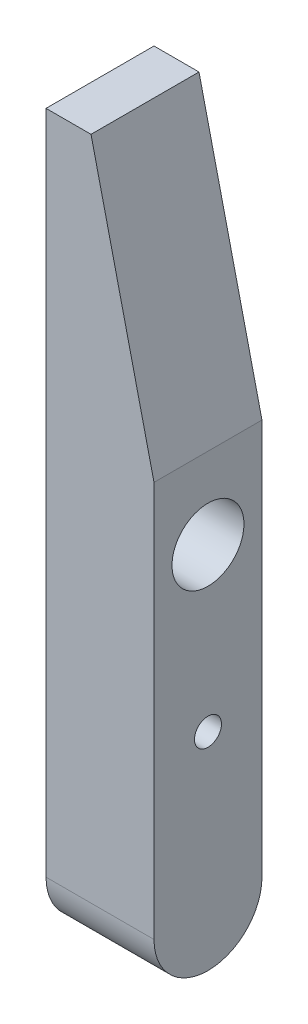
from build123d import *

# Parameters (mm, degrees)
JAW_BODY_12MM_DEPTH       = 6
END_BOSS_SKETCH_R         = 6
END_BOSS_DEPTH            = 12
CUT_4_8_SKETCH_R          = 2.4
CUT_4_8_X_6_DEPTH         = 6
TAPPED_HOLE_M8X1_25_D     = 8
TAPPED_HOLE_M8X1_25_DEPTH = 19.75
TAPPED_HOLE_M8X1_25_TIP   = 2.403442476
TAPPED_HOLE_M3X0_5_D      = 3
TAPPED_HOLE_M3X0_5_DEPTH  = 8
TAPPED_HOLE_M3X0_5_TIP    = 0.901290929


with BuildPart() as part:
    # Jaw Profile Sketch → Jaw Body 12mm (new, symmetric)
    with BuildSketch(Plane.XY):
        Polygon((0, 0), (5, 0), (12, -30), (12, -74), (0, -74), align=None)
    extrude(amount=JAW_BODY_12MM_DEPTH, both=True)

    # End Boss Sketch → End Boss (add)
    with BuildSketch(Plane.ZY):
        with Locations((0, -74)):
            Circle(END_BOSS_SKETCH_R)
    extrude(amount=-END_BOSS_DEPTH)

    # Cut Ø4.8 Sketch → Cut Ø4.8 x 6 (cut)
    with BuildSketch(Plane.ZY):
        with Locations((0, -74)):
            Circle(CUT_4_8_SKETCH_R)
    extrude(amount=-CUT_4_8_X_6_DEPTH, mode=Mode.SUBTRACT)

    # Tapped Hole M8x1.25
    with Locations(Plane(origin=(12, -39, 0), x_dir=(0, 1, 0), z_dir=(1, 0, 0))):
        with Locations((0, 0)):
            Hole(TAPPED_HOLE_M8X1_25_D / 2, depth=TAPPED_HOLE_M8X1_25_DEPTH)
            with Locations((0, 0, -(TAPPED_HOLE_M8X1_25_DEPTH + TAPPED_HOLE_M8X1_25_TIP / 2))):  # 118° drill point
                Cone(0, TAPPED_HOLE_M8X1_25_D / 2, TAPPED_HOLE_M8X1_25_TIP, mode=Mode.SUBTRACT)

    # Tapped Hole M3x0.5
    with Locations(Plane(origin=(12, -57, 0), x_dir=(0, 1, 0), z_dir=(1, 0, 0))):
        with Locations((0, 0)):
            Hole(TAPPED_HOLE_M3X0_5_D / 2, depth=TAPPED_HOLE_M3X0_5_DEPTH)
            with Locations((0, 0, -(TAPPED_HOLE_M3X0_5_DEPTH + TAPPED_HOLE_M3X0_5_TIP / 2))):  # 118° drill point
                Cone(0, TAPPED_HOLE_M3X0_5_D / 2, TAPPED_HOLE_M3X0_5_TIP, mode=Mode.SUBTRACT)


solid = part.part
